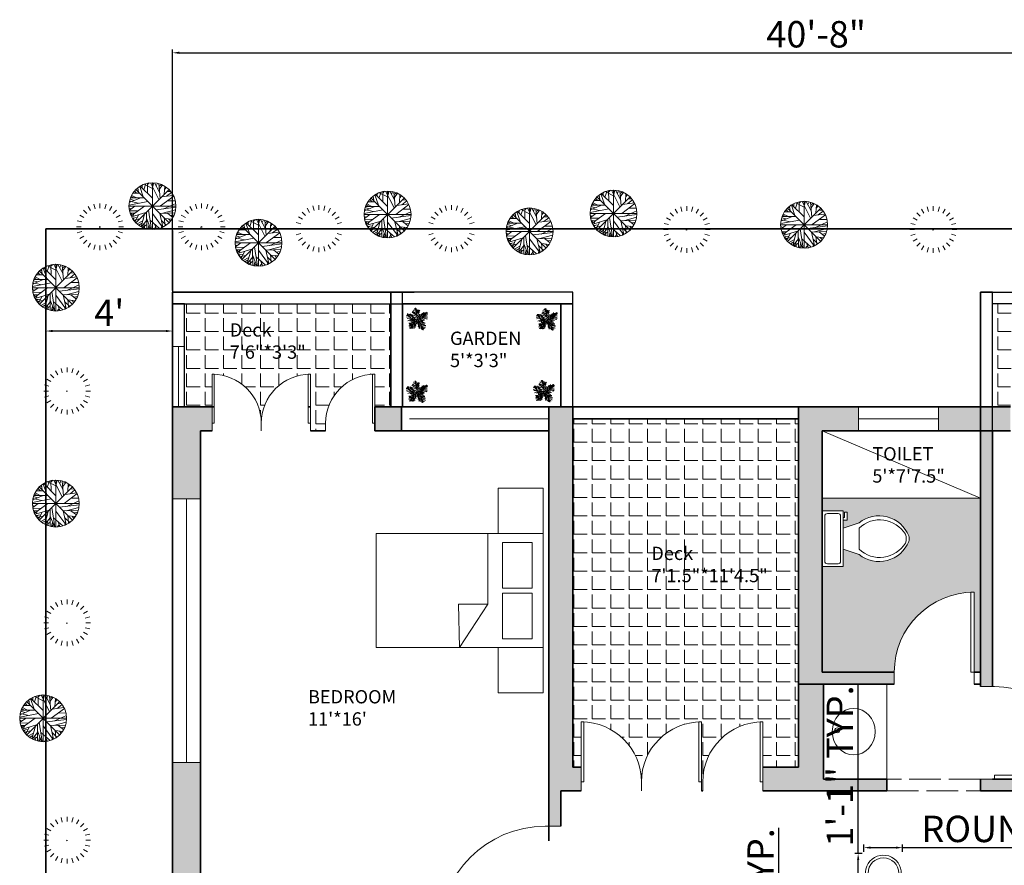
# Model space of a CAD drawing. Units: inches. Extents: x 2852 to 3654, y 1718 to 3031.
# Tile 4 of 5: x 2884 to 3257, y 2711 to 3031. Entities that reach past the tile are written whole.
import ezdxf

# ---------------------------------------------------------------- set-up
doc = ezdxf.new("R2010")
doc.units = ezdxf.units.IN
doc.linetypes.add('ACAD_ISO02W100', pattern=[15, 12, -3])
for name, color, linetype, lineweight in [('A-ANNO-DIMS', 2, 'Continuous', 18), ('A-AREA-IDEN', 7, 'Continuous', 18), ('A-DOOR', 140, 'Continuous', 18), ('A-FLOR-DECK', 52, 'Continuous', 25), ('A-FLOR-FIXT', 9, 'Continuous', 18), ('A-FLOR-PATT', 52, 'Continuous', 13), ('A-WALL-OVHD', 140, 'ACAD_ISO02W100', 18), ('A-WALL-PATT', 12, 'Continuous', 13), ('C-PROP', 7, 'Continuous', 35), ('fur', 210, 'Continuous', 18), ('tree', 74, 'Continuous', 13), ('wall', 12, 'Continuous', 35), ('window', 140, 'Continuous', 18)]:
    doc.layers.add(name, color=color, linetype=linetype, lineweight=lineweight)
doc.styles.get("Standard").update_dxf_attribs({"font": 'arial.ttf'})
doc.dimstyles.new('ISO-25', dxfattribs={"dimtxt": 10, "dimasz": 2.5, "dimexe": 1.25, "dimexo": 0.625, "dimtad": 1, "dimdec": 0, "dimlunit": 4, "dimtxsty": 'Standard', "dimcen": 2.5, "dimadec": 0, "dimazin": 0, "dimtfac": 1, "dimtdec": 0, "dimtmove": 0, "dimatfit": 3, "dimfxl": 1, "dimarcsym": 0})
pattern_1 = [(0, (0, 0), (0, 6.985), [5.08, -1.905]), (90, (0, 0), (-6.985, 4e-16), [5.08, -1.905])]

# ---------------------------------------------------------------- blocks, each defined once
blk = doc.blocks.new('*U2')
for p, q in [((0, 0), (0, -6)), ((40, 0), (40, -6))]:
    blk.add_line(p, q)
blk.add_lwpolyline([(0, 0), (0, 40), (1.75, 40), (1.75, 0)], close=True)
blk.add_arc((0, 0), 40, 0, 90)
blk = doc.blocks.new('*U4')
for p, q in [((9.5, -6), (9.5, -2)), ((-10, -8.5), (-8, -8.5)), ((-10, -9.5), (-10, -8.5)), ((-7, -9.5), (-10, -9.5)), ((-8, -8.5), (-8, -8)), ((-7, -8), (-7, -9.5)), ((-4, -8), (-6, -14)), ((4, -8), (6, -14)), ((4, -14), (-4, -14))]:
    blk.add_line(p, q)
blk.add_lwpolyline([(10.5, -8), (10.5, 0), (-10.5, 0), (-10.5, -8)], close=True)
for points in [[(-9.5, -2), (-9.5, -6)], [(8.5, -1), (-8.5, -1)], [(-8.5, -7), (8.5, -7)]]:
    blk.add_lwpolyline(points)
for centre, radius, start, end in [((-8.62, -1.88), 0.884, 81.8699, 188.1301), ((8.62, -1.88), 0.884, 351.8699, 98.1301), ((-8.62, -6.12), 0.884, 171.8699, 278.1301), ((8.62, -6.12), 0.884, 261.8699, 8.1301), ((3.52, -21.58), 12.17, 141.4691, 247.9714), ((4.2, -21.82), 11.33, 136.3677, 238.9468), ((-3.52, -21.58), 12.17, 292.0284, 38.5307), ((-4.2, -21.82), 11.33, 301.053, 43.6321), ((0, -27.88), 4, 245.7318, 294.2682), ((0, -29), 4, 254.8605, 285.1395)]:
    blk.add_arc(centre, radius, start, end)
blk = doc.blocks.new('*U8')
for p, q in [((-8.737, 47.138), (-17.069, 52.711)), ((-10.186, 53.64), (-13.084, 55.962)), ((0, 0), (-10.5, 57)), ((-9.099, 51.782), (-6.563, 55.962)), ((-7.65, 43.423), (-2.578, 49.46)), ((-47.498, 19.737), (-55.83, 18.344)), ((-40.615, 13.7), (-55.105, 10.913)), ((-31.5, 4.5), (-52.5, 25.5)), ((-33.37, 6.269), (-52.207, 5.34)), ((-48.585, 21.131), (-49.309, 29.026)), ((-28.299, 3.483), (-47.86, -5.805)), ((-43.513, 28.561), (-42.427, 15.558)), ((-38.442, 26.239), (-34.819, 7.663)), ((-21.416, 3.018), (-38.079, -8.128)), ((-35.544, 28.097), (-24.314, 3.947)), ((0, 0), (-31.5, 4.5)), ((-14.533, 2.09), (-30.834, 25.31)), ((-15.982, 2.09), (-30.11, -9.521)), ((-3.665, 19.273), (-27.574, 35.527)), ((-5.114, 28.097), (-24.676, 40.636)), ((-24.314, 23.917), (-2.941, 13.7)), ((0, 0), (-22.5, -19.5)), ((-7.288, 39.707), (-21.778, 46.673)), ((-6.563, 1.161), (-21.416, -8.128)), ((-20.691, 13.7), (-1.129, 4.876)), ((-5.839, 35.992), (4.667, 48.067)), ((-5.114, 27.632), (10.463, 46.673)), ((-2.941, 16.486), (8.652, 37.85)), ((-1.129, 6.734), (9.014, 26.704)), ((0, 0), (27, 9)), ((0, 0), (18, -22.5)), ((3.942, 1.625), (11.187, 24.381)), ((6.478, 1.625), (26.04, -8.592)), ((10.101, 3.483), (17.708, 26.239)), ((11.187, 3.483), (30.749, -5.805)), ((16.259, 5.805), (23.142, 31.348)), ((18.07, 5.805), (35.096, -3.483)), ((22.055, 7.198), (27.489, 32.277)), ((24.229, 7.663), (46.688, 1.625)), ((27, 9), (48, 36)), ((27.127, 9.056), (31.112, 35.992)), ((29.662, 12.307), (48.137, 6.269)), ((31.836, 30.883), (32.561, 16.486)), ((33.285, 16.486), (48.862, 10.913)), ((35.096, 32.741), (37.27, 22.524)), ((36.183, 19.737), (48.137, 17.88)), ((38.719, 34.134), (41.979, 28.561)), ((40.53, 25.775), (48.862, 24.846)), ((43.791, 29.954), (51.036, 30.883)), ((44.153, 36.456), (45.239, 32.741)), ((-17.431, -15.094), (-42.789, -18.809)), ((-28.299, -29.026), (-42.789, -31.348)), ((-24.314, -21.596), (-42.427, -22.06)), ((-30.834, -34.135), (-42.427, -35.528)), ((-34.457, -39.708), (-40.978, -42.494)), ((-26.849, -26.24), (-40.253, -25.775)), ((-22.5, -19.5), (-37.5, -45)), ((-32.646, -36.921), (-31.921, -44.352)), ((-15.257, -12.772), (-30.11, -12.772)), ((-29.023, -30.884), (-27.936, -43.887)), ((-25.038, -23.918), (-22.865, -45.281)), ((-20.691, -18.345), (-17.793, -44.352)), ((-6.563, -5.805), (-19.967, -9.985)), ((-17.069, -15.094), (-12.721, -40.172)), ((-13.446, -11.378), (-8.737, -32.741)), ((-9.461, -8.592), (-6.201, -23.453)), ((-4.752, -3.483), (-3.665, -14.629)), ((2.493, -3.019), (-1.491, -20.202)), ((1.769, -2.555), (24.229, -9.521)), ((5.029, -6.27), (2.131, -25.775)), ((9.014, -11.378), (3.58, -35.992)), ((14.085, -16.951), (6.478, -40.172)), ((7.565, -9.056), (32.198, -14.629)), ((18.07, -22.524), (8.289, -45.745)), ((12.274, -15.094), (36.907, -18.809)), ((20.244, -30.419), (15.897, -44.816)), ((16.259, -19.738), (36.183, -22.989)), ((18, -22.5), (27, -52.5)), ((18.433, -22.524), (40.53, -29.026)), ((19.157, -25.311), (38.719, -33.206)), ((22.78, -37.85), (19.519, -48.532)), ((21.331, -32.741), (39.081, -40.636)), ((22.78, -38.314), (34.372, -44.816)), ((24.591, -45.745), (23.142, -50.854)), ((24.591, -43.423), (30.749, -47.603)), ((26.764, -49.925), (28.213, -50.854))]:
    blk.add_line(p, q)
blk = doc.blocks.new('*U9')
for p, q in [((-25.024, 42.079), (-31.077, 52.563)), ((-13.435, 46.72), (-16.606, 58.557)), ((-1.077, 60.601), (-1.077, 48.601)), ((11.28, 46.72), (14.452, 58.557)), ((22.87, 42.079), (28.923, 52.563)), ((-42.564, 24.554), (-53.039, 30.601)), ((-34.93, 34.454), (-43.503, 43.028)), ((32.776, 34.454), (41.349, 43.028)), ((40.409, 24.554), (50.884, 30.601)), ((-61.077, 0.601), (-49.077, 0.601)), ((-47.5, 13.04), (-59.033, 16.131)), ((45.346, 13.04), (56.878, 16.131)), ((58.923, 0.601), (46.923, 0.601)), ((-47.5, -11.837), (-59.033, -14.928)), ((-42.564, -23.351), (-53.039, -29.399)), ((40.409, -23.351), (50.884, -29.399)), ((45.346, -11.837), (56.878, -14.928)), ((-34.93, -33.251), (-43.503, -41.825)), ((-25.024, -40.876), (-31.077, -51.36)), ((-13.435, -45.517), (-16.606, -57.354)), ((-1.077, -59.399), (-1.077, -47.399)), ((11.28, -45.517), (14.452, -57.354)), ((22.87, -40.876), (28.923, -51.36)), ((32.776, -33.251), (41.349, -41.825))]:
    blk.add_line(p, q)
blk.add_lwpolyline([(-1.908, 0.978), (-2.67, -0.978), (0, 0)], close=True)
blk = doc.blocks.new('*U10')
for p, q in [((-32.6092, 50.4264), (-23.2782, 23.5674)), ((-31.2008, 51.1035), (-0.2149, 20.1818)), ((-26.4472, 46.5894), (-26.2712, 53.8116)), ((-22.0458, 42.0753), (-16.5881, 57.6486)), ((-21.1656, 55.8436), (-0.0388, 45.0094)), ((-12.5388, 54.9406), (-7.9613, 59.4546)), ((-12.3627, 32.1443), (-12.5388, 58.7776)), ((-5.3205, 59.6806), (16.5105, 16.7963)), ((2.426, 54.9406), (-1.4472, 59.9056)), ((0, 59.9996), (0, -60)), ((0.4894, 48.6208), (3.6584, 59.6806)), ((18.2711, 35.5298), (5.419, 59.6806)), ((9.8203, 51.5549), (12.8133, 58.5516)), ((19.6795, 19.5047), (16.3344, 57.6486)), ((17.0387, 51.1035), (23.2006, 55.1666)), ((17.7429, 43.6552), (25.4894, 54.2636)), ((31.6513, 50.8778), (30.2429, 30.5643)), ((-53.2078, 27.4044), (-40.1797, 20.859)), ((-49.8627, 32.8214), (-32.7853, 32.8214)), ((-45.8134, 38.2383), (-40.5318, 33.0471)), ((-43.8768, 36.4326), (-44.405, 40.2696)), ((42, 42), (-42, -42)), ((42, -42), (-42, 42)), ((-40.1797, 44.558), (-36.4825, 43.2038)), ((-37.0107, 47.0408), (-35.25, 35.5298)), ((54.3626, 25.3731), (20.9119, 0.3198)), ((23.3767, 23.3417), (53.3063, 27.4044)), ((31.1232, 42.5267), (35.8767, 48.1693)), ((36.2288, 25.1474), (48.9049, 35.0784)), ((37.1091, 37.1098), (46.6161, 37.5612)), ((-59.7219, 2.8025), (-12.0106, 12.0565)), ((-32.2571, 20.6333), (-59.1937, 9.348)), ((-58.6656, 12.7336), (-35.9543, 7.5424)), ((-57.081, 17.9248), (-47.0458, 14.7649)), ((-56.0247, 20.859), (-20.8134, 20.859)), ((-54.7923, 24.4702), (-47.75, 21.0847)), ((-54.6162, -24.7335), (-20.2853, 0.0941)), ((29.3626, -6.6771), (59.4682, 7.091)), ((38.5175, 13.4107), (58.2359, 13.6364)), ((-60, 0), (60, 0)), ((-59.7219, -4.8714), (-54.2641, -6.6771)), ((-45.2853, -0.1316), (-59.0177, -10.0627)), ((-58.4895, -12.3197), (-36.4825, -11.6426)), ((-57.081, -18.4138), (-45.2853, -17.9624)), ((-52.6797, -18.188), (-55.4966, -22.0251)), ((-53.2078, -27.442), (-16.7641, -16.6081)), ((-47.2219, -19.3166), (-50.2148, -26.3135)), ((-35.9543, -22.4765), (-44.0529, -40.5329)), ((-19.9331, -20.2194), (-28.5599, -52.721)), ((-14.8275, -15.0282), (-14.6515, -57.6865)), ((-10.074, -10.0627), (-2.5036, -59.7178)), ((-0.0388, -19.0909), (25.8415, -53.8495)), ((9.2922, -9.1598), (59.6443, -2.8401)), ((18.6232, -18.6394), (26.7218, -53.3981)), ((18.7992, -18.6394), (57.3556, -17.2853)), ((26.3697, -18.4138), (58.9401, -9.8369)), ((38.1654, -18.188), (52.426, -29.0219)), ((45.9119, -24.0564), (55.595, -22.2508)), ((-38.9472, -29.0219), (-51.4472, -30.6018)), ((-46.5177, -30.1504), (-49.5106, -33.536)), ((-32.4331, -32.4075), (-48.1021, -35.5674)), ((-43.7008, -34.6645), (-46.6937, -37.373)), ((-24.6867, -37.8244), (-38.7712, -45.7241)), ((-26.2712, -43.9185), (-34.7219, -48.6583)), ((-14.6515, -36.2445), (-27.6797, -52.9467)), ((-14.6515, -47.3041), (-25.0388, -54.3009)), ((-21.5177, -45.4984), (-19.9331, -56.1065)), ((-14.6515, -32.1818), (-3.912, -59.4922)), ((-8.4895, -47.5298), (-11.4825, -58.5893)), ((-6.2008, -36.2445), (17.919, -57.0094)), ((5.9471, -46.6269), (10.5246, -58.5893)), ((22.8485, -36.4702), (35.3485, -48.4326)), ((24.7852, -44.8213), (23.0246, -54.978)), ((30.419, -30.1504), (32.3556, -50.0125)), ((31.4753, -31.279), (49.6091, -33.3103)), ((41.5105, -32.6332), (46.088, -38.0501)), ((-6.3768, -52.721), (-9.3698, -58.815)), ((8.4119, -53.1724), (3.8344, -59.4922))]:
    blk.add_line(p, q)
blk.add_circle((0, 0), 60)
blk = doc.blocks.new('*D11')
at = {"layer": 'A-ANNO-DIMS', "color": 0, "lineweight": -2, "transparency": 16777216}
for p, q in [((2942.37, 2928.32), (2942.37, 3019.61)), ((2944.87, 3018.36), (3427.45, 3018.36)), ((3429.95, 2928.32), (3429.95, 3019.61))]:
    blk.add_line(p, q, dxfattribs=at)
at = {"layer": 'A-ANNO-DIMS', "color": 0, "lineweight": 100, "transparency": 16777216}
for points in [[(2944.87, 3018.78), (2944.87, 3017.95), (2942.37, 3018.36)], [(3427.45, 3018.78), (3427.45, 3017.95), (3429.95, 3018.36)]]:
    blk.add_solid(points, dxfattribs=at)
at = {"layer": 'Defpoints', "color": 0, "lineweight": 100, "transparency": 16777216}
for p in [(3429.95, 3018.36), (2942.37, 2927.69), (3429.95, 2927.69)]:
    blk.add_point(p, dxfattribs=at)
at = {"layer": 'A-ANNO-DIMS', "color": 0, "transparency": 16777216, "insert": (3186.16, 3024.09), "char_height": 10, "attachment_point": 5}
blk.add_mtext('40\'-8"', dxfattribs=at)
blk = doc.blocks.new('*D16')
at = {"layer": 'A-ANNO-DIMS', "color": 0, "lineweight": -2, "transparency": 16777216}
for p, q in [((2894.37, 2951.07), (2894.37, 2911.69)), ((2942.37, 2951.07), (2942.37, 2911.69)), ((2939.87, 2912.94), (2896.87, 2912.94))]:
    blk.add_line(p, q, dxfattribs=at)
at = {"layer": 'A-ANNO-DIMS', "color": 0, "lineweight": 100, "transparency": 16777216}
for points in [[(2896.87, 2913.36), (2896.87, 2912.53), (2894.37, 2912.94)], [(2939.87, 2913.36), (2939.87, 2912.53), (2942.37, 2912.94)]]:
    blk.add_solid(points, dxfattribs=at)
at = {"layer": 'Defpoints', "color": 0, "lineweight": 100, "transparency": 16777216}
for p in [(2894.37, 2951.69), (2942.37, 2951.69), (2894.37, 2912.94)]:
    blk.add_point(p, dxfattribs=at)
at = {"layer": 'A-ANNO-DIMS', "color": 0, "transparency": 16777216, "insert": (2918.37, 2918.57), "char_height": 10, "attachment_point": 5}
blk.add_mtext("4'", dxfattribs=at)
blk = doc.blocks.new('BED-WITH-NIGHTSTANDS')
for p, q in [((42.38, 60.42), (42.38, 33.67)), ((42.38, 33.67), (31.23, 33.67)), ((31.23, 33.67), (31.64, 17.23)), ((31.64, 17.23), (42.38, 33.67))]:
    blk.add_line(p, q)
for points in [[(63.28, 60.42), (46.24, 60.42), (46.24, 77.65), (63.28, 77.65)], [(63.28, 60.42), (0, 60.42), (0, 17.23), (63.28, 17.23)], [(59.11, 57), (47.96, 57), (47.96, 39.69), (59.11, 39.69)], [(59.11, 37.81), (47.96, 37.81), (47.96, 20.49), (59.11, 20.49)], [(63.28, 0), (46.24, 0), (46.24, 17.23), (63.28, 17.23)]]:
    blk.add_lwpolyline(points, close=True)
blk = doc.blocks.new('CHAIR-DINING-ROUND')
for p, q in [((12.45, 4.57), (13.43, 4.36)), ((1.15, 2.01), (1.98, 2.56))]:
    blk.add_line(p, q)
blk.add_circle((6.79, 5.79), 5.79)
blk.add_arc((6.79, 5.79), 6.79, 347.8419, 213.8526)
blk = doc.blocks.new('*D29')
at = {"layer": 'A-ANNO-DIMS', "color": 0, "lineweight": -2, "transparency": 16777216}
for p, q in [((3204.28, 2715.63), (3204.28, 2718.45)), ((3206.78, 2717.2), (3216.43, 2717.2)), ((3218.93, 2715.63), (3218.93, 2718.45)), ((3218.93, 2717.2), (3408.86, 2717.2))]:
    blk.add_line(p, q, dxfattribs=at)
at = {"layer": 'A-ANNO-DIMS', "color": 0, "lineweight": 100, "transparency": 16777216}
for points in [[(3206.78, 2717.62), (3206.78, 2716.79), (3204.28, 2717.2)], [(3216.43, 2717.62), (3216.43, 2716.79), (3218.93, 2717.2)]]:
    blk.add_solid(points, dxfattribs=at)
at = {"layer": 'Defpoints', "color": 0, "lineweight": 100, "transparency": 16777216}
for p in [(3218.93, 2717.2), (3204.28, 2715.01), (3218.93, 2715.01)]:
    blk.add_point(p, dxfattribs=at)
at = {"layer": 'A-ANNO-DIMS', "color": 0, "transparency": 16777216, "insert": (3315.15, 2723), "char_height": 10, "attachment_point": 5}
blk.add_mtext('ROUND CHAIR 1\'-2 1/2" TYP.', dxfattribs=at)
blk = doc.blocks.new('*D30')
at = {"layer": 'A-ANNO-DIMS', "color": 0, "lineweight": -2, "transparency": 16777216}
for p, q in [((3202.08, 2715.01), (3202.08, 2778.77)), ((3203.66, 2715.01), (3200.83, 2715.01)), ((3202.08, 2704.26), (3202.08, 2712.51)), ((3203.66, 2701.76), (3200.83, 2701.76))]:
    blk.add_line(p, q, dxfattribs=at)
at = {"layer": 'A-ANNO-DIMS', "color": 0, "lineweight": 100, "transparency": 16777216}
for points in [[(3201.67, 2712.51), (3202.5, 2712.51), (3202.08, 2715.01)], [(3201.67, 2704.26), (3202.5, 2704.26), (3202.08, 2701.76)]]:
    blk.add_solid(points, dxfattribs=at)
at = {"layer": 'Defpoints', "color": 0, "lineweight": 100, "transparency": 16777216}
for p in [(3202.08, 2715.01), (3204.28, 2715.01), (3204.28, 2701.76)]:
    blk.add_point(p, dxfattribs=at)
at = {"layer": 'A-ANNO-DIMS', "color": 0, "transparency": 16777216, "insert": (3196.43, 2748.14), "char_height": 10, "attachment_point": 5, "rotation": 90}
blk.add_mtext('1\'-1" TYP.', dxfattribs=at)
blk = doc.blocks.new('*D32')
at = {"layer": 'A-ANNO-DIMS', "color": 0, "lineweight": -2, "transparency": 16777216}
for p, q in [((3172.08, 2660.9), (3172.08, 2724.67)), ((3170.5, 2660.9), (3173.33, 2660.9)), ((3172.08, 2650.16), (3172.08, 2658.4)), ((3170.5, 2647.66), (3173.33, 2647.66))]:
    blk.add_line(p, q, dxfattribs=at)
at = {"layer": 'A-ANNO-DIMS', "color": 0, "lineweight": 100, "transparency": 16777216}
for points in [[(3171.66, 2658.4), (3172.49, 2658.4), (3172.08, 2660.9)], [(3171.66, 2650.16), (3172.49, 2650.16), (3172.08, 2647.66)]]:
    blk.add_solid(points, dxfattribs=at)
at = {"layer": 'Defpoints', "color": 0, "lineweight": 100, "transparency": 16777216}
for p in [(3169.88, 2660.9), (3172.08, 2660.9), (3169.88, 2647.66)]:
    blk.add_point(p, dxfattribs=at)
at = {"layer": 'A-ANNO-DIMS', "color": 0, "transparency": 16777216, "insert": (3166.43, 2694.04), "char_height": 10, "attachment_point": 5, "rotation": 90}
blk.add_mtext('1\'-1" TYP.', dxfattribs=at)

msp = doc.modelspace()

# ---------------------------------------------------------------- hatches: boundary and pattern name
at = {"layer": 'A-FLOR-PATT'}
h = msp.add_hatch(dxfattribs=at)
h.set_pattern_fill('ANGLE', color=256)
h.set_pattern_definition(pattern_1)
h.paths.add_polyline_path([(3024.95, 2923.19), (2946.87, 2923.19), (2946.87, 2884.19), (2957.35, 2884.19), (2957.35, 2896.58), (2958.16, 2896.58), (2958.16, 2896.57, -0.401453), (2975.95, 2877.98, -0.401453), (2993.74, 2896.57), (2993.74, 2896.58), (2994.55, 2896.58), (2994.55, 2877.98), (2994.55, 2875.19), (3000.35, 2875.19), (3000.35, 2877.98, -0.401453), (3018.14, 2896.57), (3018.14, 2896.58), (3018.95, 2896.58), (3018.95, 2884.19), (3024.95, 2884.19)])
h.paths.add_polyline_path([(3179.45, 2879.69), (3093.95, 2879.69), (3093.95, 2747.69), (3097.2, 2747.69), (3097.2, 2764.87), (3098.19, 2764.87), (3098.19, 2764.85, -0.401453), (3119.96, 2742.11, -0.401453), (3141.73, 2764.85), (3141.73, 2764.87), (3142.73, 2764.87), (3142.73, 2742.11), (3142.73, 2738.69), (3143.2, 2738.69), (3143.2, 2742.11, -0.401453), (3164.97, 2764.85), (3164.97, 2764.87), (3165.97, 2764.87), (3165.97, 2747.69), (3179.45, 2747.69), (3179.45, 2779.19)])
h.paths.add_polyline_path([(3344.45, 2923.19), (3252.95, 2923.19), (3252.95, 2884.19), (3259.75, 2884.19), (3259.75, 2896.58), (3260.56, 2896.58), (3260.56, 2896.57, -0.401453), (3278.35, 2877.98, -0.401453), (3296.14, 2896.57), (3296.14, 2896.58), (3296.95, 2896.58), (3296.95, 2877.98), (3296.95, 2875.19), (3302.75, 2875.19), (3302.75, 2877.98, -0.401453), (3320.54, 2896.57), (3320.54, 2896.58), (3321.35, 2896.58), (3321.35, 2884.19), (3344.45, 2884.19)])
h = msp.add_hatch(dxfattribs=at)
h.set_pattern_fill('ANGLE', color=256)
h.set_pattern_definition(pattern_1)
h.paths.add_polyline_path([(3248.45, 2849.58), (3188.45, 2849.58), (3188.45, 2844.77), (3196.45, 2844.77), (3196.45, 2842.27), (3196.95, 2842.27), (3196.95, 2844.27), (3197.95, 2844.27), (3197.95, 2841.27), (3196.45, 2841.27), (3196.45, 2838.27), (3202.45, 2840.27, -0.501317), (3221.31, 2835.31, -0.132891), (3221.31, 2833.22, -0.501323), (3202.45, 2828.27), (3196.45, 2830.27), (3196.45, 2823.77), (3188.45, 2823.77), (3188.45, 2783.69), (3215.78, 2783.69), (3215.78, 2783.73, -0.401453), (3244.71, 2813.96), (3244.71, 2813.99), (3246.03, 2813.99), (3246.03, 2783.69), (3248.45, 2783.69)])
h.paths.add_polyline_path([(3420.95, 2714.69), (3324.42, 2714.69), (3324.42, 2691.18, -1), (3301.33, 2691.18), (3301.33, 2638.19), (3420.95, 2638.19)])
h.paths.add_polyline_path([(3059.57, 2647.05, -0.132891), (3061.66, 2647.05, -0.501323), (3066.62, 2628.19), (3064.62, 2622.19), (3071.12, 2622.19), (3071.12, 2614.19), (3084.95, 2614.19), (3084.95, 2678.69), (3040.14, 2678.69), (3040.14, 2677.19), (3040.14, 2637.19), (3038.39, 2637.19), (3038.39, 2637.23, -0.401453), (3000.14, 2677.19), (3000.14, 2678.69), (2994.25, 2678.69), (2994.25, 2614.19), (3050.12, 2614.19), (3050.12, 2622.19), (3052.62, 2622.19), (3052.62, 2622.69), (3050.62, 2622.69), (3050.62, 2623.69), (3053.62, 2623.69), (3053.62, 2622.19), (3056.62, 2622.19), (3054.62, 2628.19, -0.501317)])
h.paths.add_polyline_path([(3252.95, 2533.88, -0.400409), (3223.79, 2561.89), (3223.76, 2561.89), (3223.76, 2563.17), (3252.95, 2563.17), (3252.95, 2565.48), (3192.95, 2565.48), (3192.95, 2500.92), (3252.95, 2500.92)])
h.paths.add_polyline_path([(3248.45, 2338.72), (3188.45, 2338.72), (3188.45, 2271.48), (3248.45, 2271.48), (3248.45, 2273.69)])
h.paths.add_polyline_path([(3390.34, 2273.69), (3312.95, 2273.69), (3312.95, 2224.19), (3390.34, 2224.19)])
h.paths.add_polyline_path([(3365.33, 2231.19), (3382.33, 2231.19, -0.5), (3383.33, 2230.19), (3383.33, 2226.19, -0.5), (3382.33, 2225.19), (3365.33, 2225.19, -0.5), (3364.33, 2226.19), (3364.33, 2230.19, -0.5)], flags=16)
h.paths.add_polyline_path([(3372.19, 2255.72, -0.215004), (3375.48, 2255.72, -0.48008), (3377.83, 2238.19), (3369.83, 2238.19, -0.48008)], flags=16)
h.paths.add_polyline_path([(2987.37, 2220.07), (2951.37, 2220.07), (2951.37, 2095.57), (2987.37, 2095.57)])
at = {"layer": 'A-WALL-PATT'}
h = msp.add_hatch(color=256, dxfattribs=at)
h.dxf.hatch_style = 1
h.paths.add_polyline_path([(2952.95, 2875.19), (2957.35, 2875.19), (2957.35, 2877.98), (2957.35, 2884.19), (2943.95, 2884.19), (2942.37, 2884.19), (2942.37, 2849.42), (2952.95, 2849.42)])
h.paths.add_polyline_path([(2952.95, 2706.39), (2952.95, 2749.45), (2942.37, 2749.45), (2942.37, 2667.89), (2952.95, 2667.89), (2952.95, 2678.69), (3000.14, 2678.69), (3000.14, 2683.19), (2952.95, 2683.19)])
h.paths.add_polyline_path([(2951.37, 2609.69), (3089.45, 2609.69), (3089.45, 2683.19), (3089.45, 2685.28), (3084.95, 2685.28), (3084.95, 2683.19), (3084.95, 2614.19), (2952.95, 2614.19), (2952.95, 2625.26), (2942.37, 2625.26), (2942.37, 2588.19), (2951.37, 2588.19)])
h.paths.add_polyline_path([(2951.37, 2506.48), (2951.37, 2523.26), (2942.37, 2523.26), (2942.37, 2465.69), (2951.37, 2465.69), (2951.37, 2466.48)])
h.paths.add_polyline_path([(2951.37, 2367.57), (2951.37, 2370.4), (2951.37, 2376.57), (2942.37, 2376.57), (2942.37, 2312.8), (2951.37, 2312.8), (2951.37, 2320.57), (2951.37, 2324.07)])
h.paths.add_polyline_path([(3051.87, 2324.07), (3047.37, 2324.07), (2951.37, 2324.07), (2951.37, 2320.57), (3047.37, 2320.57), (3047.37, 2296.57), (3047.37, 2266.82), (3051.87, 2266.82)])
h.paths.add_polyline_path([(2951.37, 2224.57), (2942.37, 2224.57), (2942.37, 2186.63), (2951.37, 2186.63), (2951.37, 2220.07)])
h.paths.add_polyline_path([(2951.37, 2247.87), (2942.37, 2247.87), (2942.37, 2224.57), (2951.37, 2224.57)])
h.paths.add_polyline_path([(3113.37, 2224.57), (2951.37, 2224.57), (2951.37, 2220.07), (3113.37, 2220.07)])
h.paths.add_polyline_path([(2951.37, 2121.7), (2942.37, 2121.7), (2942.37, 2086.57), (3113.37, 2086.57), (3147.16, 2086.57), (3147.16, 2095.57), (3113.37, 2095.57), (2951.37, 2095.57)])
h.paths.add_polyline_path([(3429.87, 2224.19), (3276.87, 2224.19), (3276.87, 2219.69), (3420.87, 2219.69), (3420.87, 2182.43), (3429.87, 2182.43)])
h.paths.add_polyline_path([(3276.87, 2175.85), (3272.37, 2175.85), (3272.37, 2095.57), (3240.86, 2095.57), (3240.86, 2086.57), (3276.87, 2086.57)])
h.paths.add_polyline_path([(3276.87, 2224.57), (3234.52, 2224.57), (3234.52, 2220.07), (3272.37, 2220.07), (3272.37, 2215.85), (3276.87, 2215.85)])
h = msp.add_hatch(color=256, dxfattribs=at)
h.dxf.hatch_style = 1
h.paths.add_polyline_path([(3188.45, 2469.48), (3017.1, 2469.48), (3017.1, 2464.04), (3017.1, 2460.48), (3188.45, 2460.48)])
h.paths.add_polyline_path([(3420.95, 2614.19), (3299.24, 2614.19), (3299.24, 2609.69), (3420.95, 2609.69)])
h.paths.add_polyline_path([(3429.95, 2614.19), (3420.95, 2614.19), (3420.95, 2609.69), (3420.95, 2543.19), (3429.95, 2543.19)])
h.paths.add_polyline_path([(3474.95, 2646.58), (3465.95, 2646.58), (3465.95, 2614.19), (3429.95, 2614.19), (3429.95, 2605.19), (3474.95, 2605.19)])
h.paths.add_polyline_path([(3474.95, 2747.69), (3429.95, 2747.69), (3429.95, 2791.96), (3420.95, 2791.96), (3420.95, 2743.19), (3420.95, 2738.69), (3425.23, 2738.69), (3465.95, 2738.69), (3465.95, 2711.51), (3474.95, 2711.51)])
h.paths.add_polyline_path([(3420.95, 2743.19), (3301.03, 2743.19), (3252.95, 2743.19), (3248.45, 2743.19), (3248.45, 2738.69), (3349.1, 2738.69), (3420.95, 2738.69)])
h.paths.add_polyline_path([(3188.92, 2779.19), (3179.45, 2779.19), (3179.45, 2747.69), (3165.97, 2747.69), (3165.97, 2742.11), (3165.97, 2738.69), (3188.92, 2738.69), (3212.98, 2738.69), (3212.98, 2743.19), (3188.92, 2743.19)])
h.paths.add_polyline_path([(3093.95, 2879.69), (3093.95, 2884.19), (3089.45, 2884.19), (3084.95, 2884.19), (3084.95, 2875.19), (3084.95, 2725.28), (3089.45, 2725.28), (3089.45, 2738.69), (3097.2, 2738.69), (3097.2, 2742.11), (3097.2, 2747.69), (3093.95, 2747.69)])
h.paths.add_polyline_path([(3188.45, 2875.19), (3202.27, 2875.19), (3202.27, 2884.19), (3179.45, 2884.19), (3179.45, 2879.69), (3179.45, 2779.19), (3188.92, 2779.19), (3215.78, 2779.19), (3215.78, 2783.69), (3188.45, 2783.69)])
h.paths.add_polyline_path([(3248.45, 2884.19), (3232.5, 2884.19), (3232.5, 2875.19), (3248.45, 2875.19)])
h.paths.add_polyline_path([(3252.95, 2875.19), (3248.45, 2875.19), (3248.45, 2778.22), (3252.95, 2778.22)])
h.paths.add_polyline_path([(3252.95, 2884.19), (3248.45, 2884.19), (3248.45, 2875.19), (3252.95, 2875.19)])
h.paths.add_polyline_path([(3259.75, 2884.19), (3252.95, 2884.19), (3252.95, 2875.19), (3259.75, 2875.19), (3259.75, 2877.98)])
h.paths.add_polyline_path([(3329.96, 2884.19), (3321.35, 2884.19), (3321.35, 2877.98), (3321.35, 2875.19), (3329.96, 2875.19)])
h.paths.add_polyline_path([(3029.12, 2884.19), (3018.95, 2884.19), (3018.95, 2877.98), (3018.95, 2875.19), (3029.12, 2875.19)])
h.paths.add_polyline_path([(3429.95, 2884.19), (3420.95, 2884.19), (3420.95, 2875.19), (3420.95, 2843.21), (3429.95, 2843.21)])

# ---------------------------------------------------------------- linework, layer by layer
at = {"layer": 'A-FLOR-DECK'}
for p, q in [((2942.37, 2927.69), (3033.91, 2927.69)), ((2942.37, 2884.19), (2942.37, 2927.69)), ((3093.95, 2927.69), (3029.45, 2927.69)), ((3093.95, 2884.19), (3093.95, 2927.69)), ((3248.45, 2884.19), (3248.45, 2927.69)), ((3248.45, 2927.69), (3344.45, 2927.69)), ((2946.87, 2884.19), (2946.87, 2923.19)), ((2946.87, 2923.19), (3033.91, 2923.19)), ((3024.95, 2923.19), (3024.95, 2884.19)), ((3089.45, 2923.19), (3029.45, 2923.19)), ((3029.45, 2923.19), (3029.45, 2884.19)), ((3089.45, 2884.19), (3089.45, 2923.19)), ((3420.95, 2923.19), (3252.95, 2923.19)), ((3252.95, 2875.19), (3252.95, 2923.19))]:
    msp.add_line(p, q, dxfattribs=at)
for points in [[(2942.37, 2923.19), (3025.03, 2923.19), (3025.03, 2927.69), (2942.37, 2927.69)], [(3025.03, 2884.19), (3029.45, 2884.19), (3029.45, 2927.69), (3025.03, 2927.69)], [(3025.03, 2923.19), (3093.95, 2923.19), (3093.95, 2927.69), (3025.03, 2927.69)], [(3248.45, 2884.19), (3252.95, 2884.19), (3252.95, 2927.69), (3248.45, 2927.69)], [(3252.95, 2927.69), (3348.95, 2927.69), (3348.95, 2923.19), (3252.95, 2923.19)], [(2942.37, 2884.19), (2946.87, 2884.19), (2946.87, 2923.19), (2942.37, 2923.19)], [(2942.37, 2884.19), (2946.87, 2884.19), (2946.87, 2923.19), (2942.37, 2923.19)], [(3089.45, 2884.19), (3093.95, 2884.19), (3093.95, 2923.19), (3089.45, 2923.19)], [(3093.95, 2879.69), (3179.45, 2879.69), (3179.45, 2884.19), (3093.95, 2884.19)]]:
    msp.add_lwpolyline(points, close=True, dxfattribs=at)
at = {"layer": 'A-FLOR-FIXT'}
for p, q in [((3248.45, 2849.58), (3188.45, 2875.19)), ((3188.45, 2849.58), (3248.45, 2849.58)), ((3212.98, 2779.19), (3212.98, 2743.19))]:
    msp.add_line(p, q, dxfattribs=at)
msp.add_lwpolyline([(3188.92, 2779.19), (3212.98, 2779.19), (3212.98, 2743.19), (3188.92, 2743.19)], close=True, dxfattribs=at)
msp.add_circle((3194.16, 2761.66), 0.925, dxfattribs=at)
msp.add_ellipse((3200.42, 2761.15), major_axis=(0, 8.82), ratio=0.923077, dxfattribs=at)
at = {"layer": 'A-WALL-OVHD'}
msp.add_lwpolyline([(3212.98, 2738.69), (3248.45, 2738.69), (3248.45, 2743.19), (3212.98, 2743.19)], close=True, dxfattribs=at)
at = {"layer": 'C-PROP'}
for p, q in [((2894.37, 2927.69), (2894.37, 2951.69)), ((2894.37, 2951.69), (3474.95, 2951.69)), ((2894.37, 1890.07), (2894.37, 2927.69))]:
    msp.add_line(p, q, dxfattribs=at)
at = {"layer": 'wall'}
for p, q in [((2942.37, 2224.57), (2942.37, 2884.19)), ((2942.37, 2884.19), (2945.11, 2884.19)), ((2958.16, 2884.19), (2943.95, 2884.19)), ((2994.55, 2884.19), (2993.74, 2884.19)), ((3084.95, 2884.19), (3018.95, 2884.19)), ((3029.12, 2884.19), (3034.18, 2884.19)), ((3084.95, 2879.69), (3084.95, 2884.19)), ((3084.95, 2884.19), (3093.95, 2884.19)), ((3179.45, 2884.19), (3093.95, 2884.19)), ((3093.95, 2884.19), (3093.95, 2879.69)), ((3248.45, 2884.19), (3179.45, 2884.19)), ((3179.45, 2884.19), (3179.45, 2779.19)), ((3248.45, 2884.19), (3248.45, 2778.22)), ((3259.75, 2884.19), (3248.45, 2884.19)), ((3084.95, 2879.69), (3084.95, 2743.19)), ((3179.45, 2879.69), (3093.95, 2879.69)), ((3093.95, 2879.69), (3093.95, 2747.69)), ((2952.95, 2683.19), (2952.95, 2875.19)), ((2957.35, 2875.19), (2952.95, 2875.19)), ((3000.35, 2875.19), (2994.55, 2875.19)), ((3084.95, 2875.19), (3018.95, 2875.19)), ((3029.12, 2875.19), (3036.33, 2875.19)), ((3084.95, 2875.19), (3084.95, 2725.28)), ((3248.45, 2875.19), (3188.45, 2875.19)), ((3188.45, 2875.19), (3188.45, 2783.69)), ((3252.95, 2875.19), (3248.45, 2875.19)), ((3252.95, 2875.19), (3252.95, 2778.22)), ((3259.75, 2875.19), (3252.95, 2875.19)), ((3188.45, 2783.69), (3215.78, 2783.69)), ((3246.03, 2783.69), (3248.45, 2783.69)), ((3179.45, 2779.19), (3215.78, 2779.19)), ((3179.45, 2779.19), (3179.45, 2747.69)), ((3188.92, 2779.19), (3188.92, 2743.19)), ((3246.03, 2779.19), (3248.45, 2779.19)), ((3093.95, 2747.69), (3097.2, 2747.69)), ((3165.97, 2747.69), (3179.45, 2747.69)), ((3084.95, 2743.19), (3084.95, 2719.75)), ((3188.92, 2743.19), (3212.98, 2743.19)), ((3212.98, 2743.19), (3212.98, 2738.69)), ((3248.45, 2743.19), (3248.45, 2738.69)), ((3252.95, 2743.19), (3349.1, 2743.19)), ((3089.45, 2738.69), (3097.2, 2738.69)), ((3089.45, 2738.69), (3089.45, 2725.28)), ((3142.73, 2738.69), (3143.2, 2738.69)), ((3165.97, 2738.69), (3188.92, 2738.69)), ((3179.45, 2738.69), (3212.98, 2738.69)), ((3248.45, 2738.69), (3349.1, 2738.69))]:
    msp.add_line(p, q, dxfattribs=at)
msp.add_lwpolyline([(3018.95, 2875.19), (3029.12, 2875.19), (3029.12, 2884.19), (3018.95, 2884.19)], close=True, dxfattribs=at)
msp.add_lwpolyline([(3018.95, 2875.19), (3029.12, 2875.19), (3029.12, 2884.19), (3018.95, 2884.19)], close=True, dxfattribs=at)
for points in [[(3021.95, 2884.19), (3032.17, 2884.19)], [(3032.17, 2875.19), (3021.95, 2875.19)]]:
    msp.add_lwpolyline(points, dxfattribs=at)
at = {"layer": 'window'}
for p, q in [((2944.62, 2884.19), (2944.62, 2907.12)), ((3032.17, 2879.69), (3084.95, 2879.69)), ((3202.27, 2879.69), (3232.5, 2879.69)), ((2947.66, 2749.45), (2947.66, 2849.42))]:
    msp.add_line(p, q, dxfattribs=at)
for points in [[(2942.37, 2884.19), (2946.87, 2884.19), (2946.87, 2907.12), (2942.37, 2907.12)], [(3202.27, 2875.19), (3232.5, 2875.19), (3232.5, 2884.19), (3202.27, 2884.19)], [(2942.37, 2749.45), (2952.95, 2749.45), (2952.95, 2849.42), (2942.37, 2849.42)]]:
    msp.add_lwpolyline(points, close=True, dxfattribs=at)
msp.add_lwpolyline([(3032.17, 2884.19), (3084.95, 2884.19), (3084.95, 2875.19), (3032.17, 2875.19)], dxfattribs=at)

# ---------------------------------------------------------------- block references
at = {"layer": 'A-DOOR'}
for p, xscale, yscale, zscale in [((2957.35, 2877.98), 0.4650478663129195, 0.4650478663129195, 0.4650478663129195), ((2994.55, 2877.98), -0.4650478663129195, 0.4650478663129195, 0.4650478663129195), ((3018.95, 2877.98), -0.4650478663129195, 0.4650478663129195, 0.4650478663129195), ((3246.03, 2783.73), -0.7564018755985065, 0.7564018755985065, 0.7564018755985065), ((3097.2, 2742.11), 0.569115171360034, 0.569115171360034, 0.569115171360034), ((3142.73, 2742.11), -0.569115171360034, 0.569115171360034, 0.569115171360034), ((3165.97, 2742.11), -0.569115171360034, 0.569115171360034, 0.569115171360034)]:
    msp.add_blockref('*U2', p, dxfattribs=dict(at, xscale=xscale, yscale=yscale, zscale=zscale))
at = {"layer": 'A-DOOR', "xscale": -0.8757866022194583, "yscale": 0.8757866022194583, "zscale": 0.8757866022194583, "rotation": 270}
msp.add_blockref('*U2', (3253.71, 2743.19), dxfattribs=at)
at = {"layer": 'A-DOOR', "rotation": 90}
msp.add_blockref('*U2', (3083.45, 2685.28), dxfattribs=at)
at = {"layer": 'A-FLOR-FIXT', "xscale": -1, "rotation": 90}
msp.add_blockref('*U4', (3188.45, 2834.27), dxfattribs=at)
at = {"layer": 'fur'}
for name, p in [('BED-WITH-NIGHTSTANDS', (3019.43, 2775.81)), ('CHAIR-DINING-ROUND', (3204.85, 2701.76))]:
    msp.add_blockref(name, p, dxfattribs=at)
at = {"layer": 'tree'}
for name, p, xscale, yscale, zscale in [('*U10', (2934.72, 2960.27), 0.1480989313836924, 0.1480989313836924, 0.1480989313836924), ('*U10', (3023.81, 2957.08), 0.1480989313836924, 0.1480989313836924, 0.1480989313836924), ('*U10', (3109.4, 2957.48), 0.1480989313836924, 0.1480989313836924, 0.1480989313836924), ('*U10', (3181.6, 2953.21), 0.1480989313836924, 0.1480989313836924, 0.1480989313836924), ('*U9', (2915.01, 2952.35), 0.1480989313836924, 0.1480989313836924, 0.1480989313836924), ('*U9', (2953.51, 2952.35), 0.1480989313836924, 0.1480989313836924, 0.1480989313836924), ('*U9', (2997.94, 2951.66), 0.1480989313836924, 0.1480989313836924, 0.1480989313836924), ('*U9', (3048.14, 2951.66), 0.1480989313836924, 0.1480989313836924, 0.1480989313836924), ('*U10', (3077.6, 2950.69), 0.1480989313836924, 0.1480989313836924, 0.1480989313836924), ('*U9', (3137.32, 2951.34), 0.1480989313836924, 0.1480989313836924, 0.1480989313836924), ('*U9', (3230.72, 2951.34), 0.1480989313836924, 0.1480989313836924, 0.1480989313836924), ('*U10', (2974.89, 2946.38), 0.1480989313836924, 0.1480989313836924, 0.1480989313836924), ('*U10', (2898.14, 2929.37), 0.1480989313836924, 0.1480989313836924, 0.1480989313836924), ('*U8', (3035.18, 2917.31), 0.0764996412196377, 0.0764996412196377, 0.0764996412196377), ('*U8', (3084.33, 2917.16), 0.0764996412196377, 0.0764996412196377, 0.0764996412196377), ('*U9', (2902.57, 2890.13), 0.1480989313836924, 0.1480989313836924, 0.1480989313836924), ('*U8', (3035.12, 2889.72), 0.0764996412196377, 0.0764996412196377, 0.0764996412196377), ('*U8', (3083.18, 2889.98), 0.0764996412196377, 0.0764996412196377, 0.0764996412196377), ('*U10', (2898.14, 2847.57), 0.1480989313836924, 0.1480989313836924, 0.1480989313836924), ('*U9', (2902.57, 2802.28), 0.1480989313836924, 0.1480989313836924, 0.1480989313836924), ('*U10', (2893.32, 2766.2), 0.1480989313836924, 0.1480989313836924, 0.1480989313836924), ('*U9', (2902.57, 2719.95), 0.1480989313836924, 0.1480989313836924, 0.1480989313836924)]:
    msp.add_blockref(name, p, dxfattribs=dict(at, xscale=xscale, yscale=yscale, zscale=zscale))

# ---------------------------------------------------------------- texts
at = {"layer": 'A-AREA-IDEN', "attachment_point": 1}
for s, insert, char_height in [('Deck\\P7\'6"*3\'3"', (2964, 2915.88), 5.041), ('GARDEN\\P5\'*3\'3"', (3047.46, 2912.72), 5.041), ('TOILET\\P5\'*7\'7.5"', (3207.45, 2868.94), 5.041), ('Deck\\P7\'1.5"*11\'4.5"', (3123.73, 2831.23), 5.0412), ("BEDROOM\\P11'*16'", (2993.66, 2776.89), 5.041)]:
    msp.add_mtext_dynamic_manual_height_columns(s, width=98.3816, gutter_width=25.21, heights=[0], dxfattribs=dict(at, insert=insert, char_height=char_height))

# ---------------------------------------------------------------- dimensions: what is measured, and where the dimension line sits
at = {"layer": 'A-ANNO-DIMS'}
for base, p1, p2, picture, middle in [((3429.95, 3018.36), (2942.37, 2927.69), (3429.95, 2927.69), '*D11', (3186.16, 3024.09)), ((2894.37, 2912.94), (2942.37, 2951.69), (2894.37, 2951.69), '*D16', (2918.37, 2918.57))]:
    dim = msp.add_linear_dim(base=base, p1=p1, p2=p2, dimstyle='ISO-25', override={"dimclrd": 0, "dimclre": 0, "dimclrt": 0}, dxfattribs=at)
    dim.commit()
    dim.dimension.update_dxf_attribs({"geometry": picture, "text_midpoint": middle})
for base, p1, p2, picture, middle in [((3202.0837, 2715.0052), (3204.2806, 2701.7636), (3204.2806, 2715.0052), '*D30', (3196.4349, 2748.1371)), ((3172.08, 2660.9), (3169.88, 2647.66), (3169.88, 2660.9), '*D32', (3166.43, 2694.04))]:
    dim = msp.add_linear_dim(base=base, p1=p1, p2=p2, angle=90, text='<> TYP.', dimstyle='ISO-25', override={"dimdec": 1, "dimlfac": 1, "dimrnd": 0, "dimzin": 1, "dimdsep": 46, "dimlunit": 4, "dimfrac": 2}, dxfattribs=at)
    dim.commit()
    dim.dimension.update_dxf_attribs({"geometry": picture, "text_midpoint": middle})
dim = msp.add_linear_dim(base=(3218.9266, 2717.2021), p1=(3204.2806, 2715.0052), p2=(3218.9266, 2715.0052), text='ROUND CHAIR <> TYP.', dimstyle='ISO-25', override={"dimdec": 1, "dimlfac": 1, "dimrnd": 0, "dimzin": 1, "dimdsep": 46, "dimlunit": 4, "dimfrac": 2}, dxfattribs=at)
dim.commit()
dim.dimension.update_dxf_attribs({"geometry": '*D29', "text_midpoint": (3315.145, 2723.0011)})

doc.saveas('drawing.dxf')
